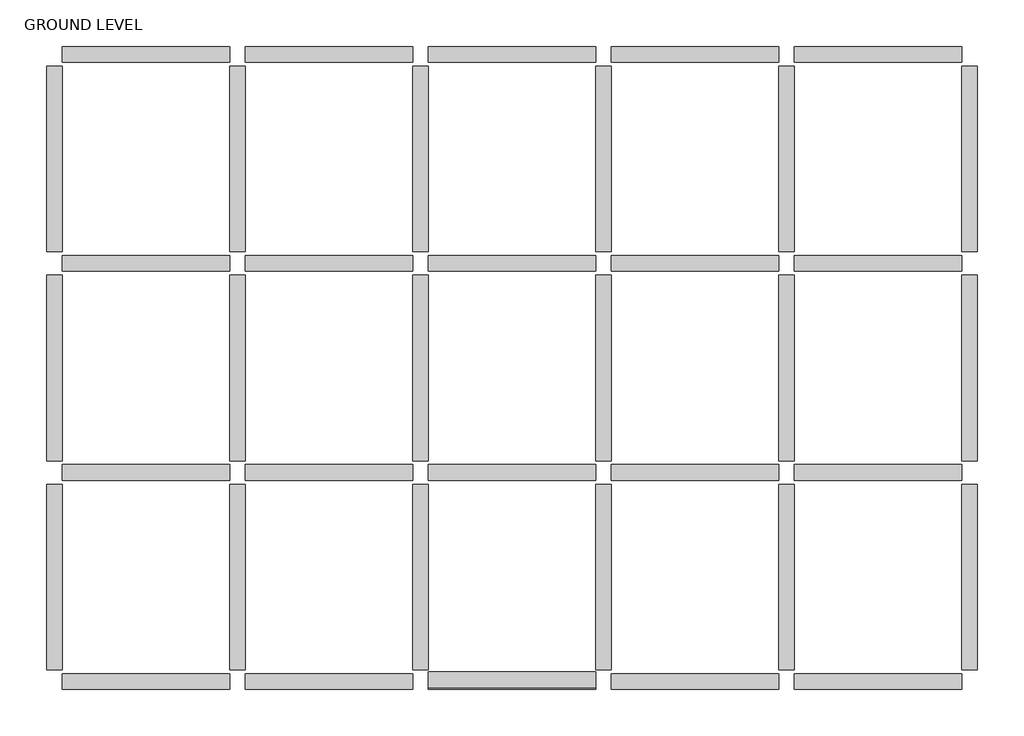
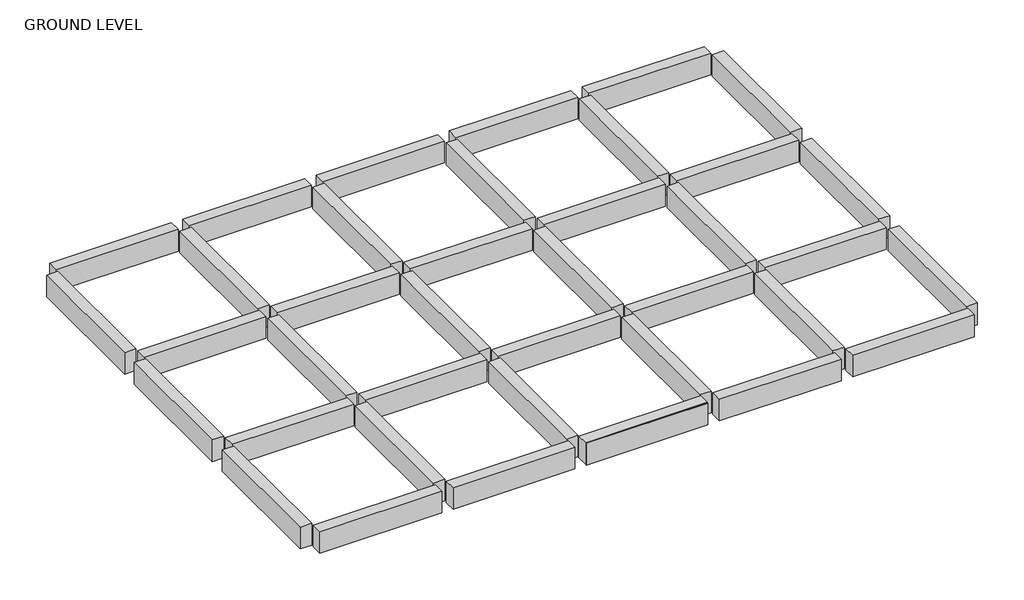
# One storey: 39 beams.
"""IFC4 building model written with IfcOpenShell, lengths in millimetres."""

from ifc_helpers import new_model, si_unit, frame, origin, place, context, project, spatial, polyline, outline, extrude, element, save

model = new_model("IFC4")

# Units and contexts
model_context = context("Model", 3, world=origin())
ifc_project = project(units=[si_unit("LENGTHUNIT", "METRE", prefix="MILLI")], contexts=[model_context])

# Site, building, storey
site = spatial("IfcSite", under=ifc_project)
building = spatial("IfcBuilding", under=site)
storey = spatial("IfcBuildingStorey", under=building, Name="GROUND LEVEL", Elevation=0.0)

# Beams
placement = place(None, origin())
element("IfcBeam", 1, ObjectType="M_Concrete-Rectangular Beam : 300 x 600mm", at=placement, inside=storey, context=model_context, shape_type="SweptSolid", body=[
    extrude(outline(polyline([(-8225.6838695, 13443.2036311), (-8525.6838695, 13443.2036311), (-8525.6838695, 16993.2036311), (-8225.6838695, 16993.2036311), (-8225.6838695, 13443.2036311)])), frame((0.0, 0.0, -600.0), z_axis=(0.0, 0.0, 1.0), x_axis=(1.0, 0.0, 0.0)), (0.0, 0.0, 1.0), 600.0),
])
element("IfcBeam", 2, ObjectType="M_Concrete-Rectangular Beam : 300 x 600mm", at=placement, inside=storey, context=model_context, shape_type="SweptSolid", body=[
    extrude(outline(polyline([(-8525.6838695, 12993.2036311), (-8225.6838695, 12993.2036311), (-8225.6838695, 9443.2036311), (-8525.6838695, 9443.2036311), (-8525.6838695, 12993.2036311)])), frame((0.0, 0.0, -600.0), z_axis=(0.0, 0.0, 1.0), x_axis=(1.0, 0.0, 0.0)), (0.0, 0.0, 1.0), 600.0),
])
element("IfcBeam", 3, ObjectType="M_Concrete-Rectangular Beam : 300 x 600mm", at=placement, inside=storey, context=model_context, shape_type="SweptSolid", body=[
    extrude(outline(polyline([(-8225.6838695, 5443.2036311), (-8525.6838695, 5443.2036311), (-8525.6838695, 8993.2036311), (-8225.6838695, 8993.2036311), (-8225.6838695, 5443.2036311)])), frame((0.0, 0.0, -600.0), z_axis=(0.0, 0.0, 1.0), x_axis=(1.0, 0.0, 0.0)), (0.0, 0.0, 1.0), 600.0),
])
element("IfcBeam", 4, ObjectType="M_Concrete-Rectangular Beam : 300 x 600mm", at=placement, inside=storey, context=model_context, shape_type="SweptSolid", body=[
    extrude(outline(polyline([(-5025.6838695, 5368.2036311), (-5025.6838695, 5068.2036311), (-8225.6838695, 5068.2036311), (-8225.6838695, 5368.2036311), (-5025.6838695, 5368.2036311)])), frame((0.0, 0.0, -600.0), z_axis=(0.0, 0.0, 1.0), x_axis=(1.0, 0.0, 0.0)), (0.0, 0.0, 1.0), 600.0),
])
element("IfcBeam", 5, ObjectType="M_Concrete-Rectangular Beam : 300 x 600mm", at=placement, inside=storey, context=model_context, shape_type="SweptSolid", body=[
    extrude(outline(polyline([(-1525.6838695, 5368.2036311), (-1525.6838695, 5068.2036311), (-4725.6838695, 5068.2036311), (-4725.6838695, 5368.2036311), (-1525.6838695, 5368.2036311)])), frame((0.0, 0.0, -600.0), z_axis=(0.0, 0.0, 1.0), x_axis=(1.0, 0.0, 0.0)), (0.0, 0.0, 1.0), 600.0),
])
element("IfcBeam", 6, ObjectType="M_Concrete-Rectangular Beam : 300 x 600mm", at=placement, inside=storey, context=model_context, shape_type="SweptSolid", body=[
    extrude(outline(polyline([(1974.3161305, 5399.3942253), (1974.3161305, 5099.3942253), (-1225.6838695, 5099.3942253), (-1225.6838695, 5399.3942253), (1974.3161305, 5399.3942253)])), frame((0.0, 0.0, -600.0), z_axis=(0.0, 0.0, 1.0), x_axis=(1.0, 0.0, 0.0)), (0.0, 0.0, 1.0), 600.0),
])
element("IfcBeam", 7, ObjectType="M_Concrete-Rectangular Beam : 300 x 600mm", at=placement, inside=storey, context=model_context, shape_type="SweptSolid", body=[
    extrude(outline(polyline([(-5025.6838695, 8993.2036311), (-4725.6838695, 8993.2036311), (-4725.6838695, 5443.2036311), (-5025.6838695, 5443.2036311), (-5025.6838695, 8993.2036311)])), frame((0.0, 0.0, -600.0), z_axis=(0.0, 0.0, 1.0), x_axis=(1.0, 0.0, 0.0)), (0.0, 0.0, 1.0), 600.0),
])
element("IfcBeam", 8, ObjectType="M_Concrete-Rectangular Beam : 300 x 600mm", at=placement, inside=storey, context=model_context, shape_type="SweptSolid", body=[
    extrude(outline(polyline([(-5025.6838695, 12993.2036311), (-4725.6838695, 12993.2036311), (-4725.6838695, 9443.2036311), (-5025.6838695, 9443.2036311), (-5025.6838695, 12993.2036311)])), frame((0.0, 0.0, -600.0), z_axis=(0.0, 0.0, 1.0), x_axis=(1.0, 0.0, 0.0)), (0.0, 0.0, 1.0), 600.0),
])
element("IfcBeam", 9, ObjectType="M_Concrete-Rectangular Beam : 300 x 600mm", at=placement, inside=storey, context=model_context, shape_type="SweptSolid", body=[
    extrude(outline(polyline([(-5025.6838695, 16993.2036311), (-4725.6838695, 16993.2036311), (-4725.6838695, 13443.2036311), (-5025.6838695, 13443.2036311), (-5025.6838695, 16993.2036311)])), frame((0.0, 0.0, -600.0), z_axis=(0.0, 0.0, 1.0), x_axis=(1.0, 0.0, 0.0)), (0.0, 0.0, 1.0), 600.0),
])
element("IfcBeam", 10, ObjectType="M_Concrete-Rectangular Beam : 300 x 600mm", at=placement, inside=storey, context=model_context, shape_type="SweptSolid", body=[
    extrude(outline(polyline([(-1525.6838695, 8993.2036311), (-1225.6838695, 8993.2036311), (-1225.6838695, 5443.2036311), (-1525.6838695, 5443.2036311), (-1525.6838695, 8993.2036311)])), frame((0.0, 0.0, -600.0), z_axis=(0.0, 0.0, 1.0), x_axis=(1.0, 0.0, 0.0)), (0.0, 0.0, 1.0), 600.0),
])
element("IfcBeam", 11, ObjectType="M_Concrete-Rectangular Beam : 300 x 600mm", at=placement, inside=storey, context=model_context, shape_type="SweptSolid", body=[
    extrude(outline(polyline([(-1525.6838695, 12993.2036311), (-1225.6838695, 12993.2036311), (-1225.6838695, 9443.2036311), (-1525.6838695, 9443.2036311), (-1525.6838695, 12993.2036311)])), frame((0.0, 0.0, -600.0), z_axis=(0.0, 0.0, 1.0), x_axis=(1.0, 0.0, 0.0)), (0.0, 0.0, 1.0), 600.0),
])
element("IfcBeam", 12, ObjectType="M_Concrete-Rectangular Beam : 300 x 600mm", at=placement, inside=storey, context=model_context, shape_type="SweptSolid", body=[
    extrude(outline(polyline([(-1525.6838695, 16993.2036311), (-1225.6838695, 16993.2036311), (-1225.6838695, 13443.2036311), (-1525.6838695, 13443.2036311), (-1525.6838695, 16993.2036311)])), frame((0.0, 0.0, -600.0), z_axis=(0.0, 0.0, 1.0), x_axis=(1.0, 0.0, 0.0)), (0.0, 0.0, 1.0), 600.0),
])
element("IfcBeam", 13, ObjectType="M_Concrete-Rectangular Beam : 300 x 600mm", at=placement, inside=storey, context=model_context, shape_type="SweptSolid", body=[
    extrude(outline(polyline([(1974.3161305, 8993.2036311), (2274.3161305, 8993.2036311), (2274.3161305, 5443.2036311), (1974.3161305, 5443.2036311), (1974.3161305, 8993.2036311)])), frame((0.0, 0.0, -600.0), z_axis=(0.0, 0.0, 1.0), x_axis=(1.0, 0.0, 0.0)), (0.0, 0.0, 1.0), 600.0),
])
element("IfcBeam", 14, ObjectType="M_Concrete-Rectangular Beam : 300 x 600mm", at=placement, inside=storey, context=model_context, shape_type="SweptSolid", body=[
    extrude(outline(polyline([(1974.3161305, 12993.2036311), (2274.3161305, 12993.2036311), (2274.3161305, 9443.2036311), (1974.3161305, 9443.2036311), (1974.3161305, 12993.2036311)])), frame((0.0, 0.0, -600.0), z_axis=(0.0, 0.0, 1.0), x_axis=(1.0, 0.0, 0.0)), (0.0, 0.0, 1.0), 600.0),
])
element("IfcBeam", 15, ObjectType="M_Concrete-Rectangular Beam : 300 x 600mm", at=placement, inside=storey, context=model_context, shape_type="SweptSolid", body=[
    extrude(outline(polyline([(1974.3161305, 16993.2036311), (2274.3161305, 16993.2036311), (2274.3161305, 13443.2036311), (1974.3161305, 13443.2036311), (1974.3161305, 16993.2036311)])), frame((0.0, 0.0, -600.0), z_axis=(0.0, 0.0, 1.0), x_axis=(1.0, 0.0, 0.0)), (0.0, 0.0, 1.0), 600.0),
])
element("IfcBeam", 16, ObjectType="M_Concrete-Rectangular Beam : 300 x 600mm", at=placement, inside=storey, context=model_context, shape_type="SweptSolid", body=[
    extrude(outline(polyline([(5474.3161305, 8993.2036311), (5774.3161305, 8993.2036311), (5774.3161305, 5443.2036311), (5474.3161305, 5443.2036311), (5474.3161305, 8993.2036311)])), frame((0.0, 0.0, -600.0), z_axis=(0.0, 0.0, 1.0), x_axis=(1.0, 0.0, 0.0)), (0.0, 0.0, 1.0), 600.0),
])
element("IfcBeam", 17, ObjectType="M_Concrete-Rectangular Beam : 300 x 600mm", at=placement, inside=storey, context=model_context, shape_type="SweptSolid", body=[
    extrude(outline(polyline([(5474.3161305, 12993.2036311), (5774.3161305, 12993.2036311), (5774.3161305, 9443.2036311), (5474.3161305, 9443.2036311), (5474.3161305, 12993.2036311)])), frame((0.0, 0.0, -600.0), z_axis=(0.0, 0.0, 1.0), x_axis=(1.0, 0.0, 0.0)), (0.0, 0.0, 1.0), 600.0),
])
element("IfcBeam", 18, ObjectType="M_Concrete-Rectangular Beam : 300 x 600mm", at=placement, inside=storey, context=model_context, shape_type="SweptSolid", body=[
    extrude(outline(polyline([(5474.3161305, 16993.2036311), (5774.3161305, 16993.2036311), (5774.3161305, 13443.2036311), (5474.3161305, 13443.2036311), (5474.3161305, 16993.2036311)])), frame((0.0, 0.0, -600.0), z_axis=(0.0, 0.0, 1.0), x_axis=(1.0, 0.0, 0.0)), (0.0, 0.0, 1.0), 600.0),
])
element("IfcBeam", 19, ObjectType="M_Concrete-Rectangular Beam : 300 x 600mm", at=placement, inside=storey, context=model_context, shape_type="SweptSolid", body=[
    extrude(outline(polyline([(8974.3161305, 8993.2036311), (9274.3161305, 8993.2036311), (9274.3161305, 5443.2036311), (8974.3161305, 5443.2036311), (8974.3161305, 8993.2036311)])), frame((0.0, 0.0, -600.0), z_axis=(0.0, 0.0, 1.0), x_axis=(1.0, 0.0, 0.0)), (0.0, 0.0, 1.0), 600.0),
])
element("IfcBeam", 20, ObjectType="M_Concrete-Rectangular Beam : 300 x 600mm", at=placement, inside=storey, context=model_context, shape_type="SweptSolid", body=[
    extrude(outline(polyline([(8974.3161305, 12993.2036311), (9274.3161305, 12993.2036311), (9274.3161305, 9443.2036311), (8974.3161305, 9443.2036311), (8974.3161305, 12993.2036311)])), frame((0.0, 0.0, -600.0), z_axis=(0.0, 0.0, 1.0), x_axis=(1.0, 0.0, 0.0)), (0.0, 0.0, 1.0), 600.0),
])
element("IfcBeam", 21, ObjectType="M_Concrete-Rectangular Beam : 300 x 600mm", at=placement, inside=storey, context=model_context, shape_type="SweptSolid", body=[
    extrude(outline(polyline([(8974.3161305, 16993.2036311), (9274.3161305, 16993.2036311), (9274.3161305, 13443.2036311), (8974.3161305, 13443.2036311), (8974.3161305, 16993.2036311)])), frame((0.0, 0.0, -600.0), z_axis=(0.0, 0.0, 1.0), x_axis=(1.0, 0.0, 0.0)), (0.0, 0.0, 1.0), 600.0),
])
element("IfcBeam", 22, ObjectType="M_Concrete-Rectangular Beam : 300 x 600mm", at=placement, inside=storey, context=model_context, shape_type="SweptSolid", body=[
    extrude(outline(polyline([(-8225.6838695, 17068.2036311), (-8225.6838695, 17368.2036311), (-5025.6838695, 17368.2036311), (-5025.6838695, 17068.2036311), (-8225.6838695, 17068.2036311)])), frame((0.0, 0.0, -600.0), z_axis=(0.0, 0.0, 1.0), x_axis=(1.0, 0.0, 0.0)), (0.0, 0.0, 1.0), 600.0),
])
element("IfcBeam", 23, ObjectType="M_Concrete-Rectangular Beam : 300 x 600mm", at=placement, inside=storey, context=model_context, shape_type="SweptSolid", body=[
    extrude(outline(polyline([(-4725.6838695, 17068.2036311), (-4725.6838695, 17368.2036311), (-1525.6838695, 17368.2036311), (-1525.6838695, 17068.2036311), (-4725.6838695, 17068.2036311)])), frame((0.0, 0.0, -600.0), z_axis=(0.0, 0.0, 1.0), x_axis=(1.0, 0.0, 0.0)), (0.0, 0.0, 1.0), 600.0),
])
element("IfcBeam", 24, ObjectType="M_Concrete-Rectangular Beam : 300 x 600mm", at=placement, inside=storey, context=model_context, shape_type="SweptSolid", body=[
    extrude(outline(polyline([(-1225.6838695, 17068.2036311), (-1225.6838695, 17368.2036311), (1974.3161305, 17368.2036311), (1974.3161305, 17068.2036311), (-1225.6838695, 17068.2036311)])), frame((0.0, 0.0, -600.0), z_axis=(0.0, 0.0, 1.0), x_axis=(1.0, 0.0, 0.0)), (0.0, 0.0, 1.0), 600.0),
])
element("IfcBeam", 25, ObjectType="M_Concrete-Rectangular Beam : 300 x 600mm", at=placement, inside=storey, context=model_context, shape_type="SweptSolid", body=[
    extrude(outline(polyline([(2274.3161305, 17068.2036311), (2274.3161305, 17368.2036311), (5474.3161305, 17368.2036311), (5474.3161305, 17068.2036311), (2274.3161305, 17068.2036311)])), frame((0.0, 0.0, -600.0), z_axis=(0.0, 0.0, 1.0), x_axis=(1.0, 0.0, 0.0)), (0.0, 0.0, 1.0), 600.0),
])
element("IfcBeam", 26, ObjectType="M_Concrete-Rectangular Beam : 300 x 600mm", at=placement, inside=storey, context=model_context, shape_type="SweptSolid", body=[
    extrude(outline(polyline([(5774.3161305, 17068.2036311), (5774.3161305, 17368.2036311), (8974.3161305, 17368.2036311), (8974.3161305, 17068.2036311), (5774.3161305, 17068.2036311)])), frame((0.0, 0.0, -600.0), z_axis=(0.0, 0.0, 1.0), x_axis=(1.0, 0.0, 0.0)), (0.0, 0.0, 1.0), 600.0),
])
element("IfcBeam", 27, ObjectType="M_Concrete-Rectangular Beam : 300 x 600mm", at=placement, inside=storey, context=model_context, shape_type="SweptSolid", body=[
    extrude(outline(polyline([(-5025.6838695, 13368.2036311), (-5025.6838695, 13068.2036311), (-8225.6838695, 13068.2036311), (-8225.6838695, 13368.2036311), (-5025.6838695, 13368.2036311)])), frame((0.0, 0.0, -600.0), z_axis=(0.0, 0.0, 1.0), x_axis=(1.0, 0.0, 0.0)), (0.0, 0.0, 1.0), 600.0),
])
element("IfcBeam", 28, ObjectType="M_Concrete-Rectangular Beam : 300 x 600mm", at=placement, inside=storey, context=model_context, shape_type="SweptSolid", body=[
    extrude(outline(polyline([(-1525.6838695, 13368.2036311), (-1525.6838695, 13068.2036311), (-4725.6838695, 13068.2036311), (-4725.6838695, 13368.2036311), (-1525.6838695, 13368.2036311)])), frame((0.0, 0.0, -600.0), z_axis=(0.0, 0.0, 1.0), x_axis=(1.0, 0.0, 0.0)), (0.0, 0.0, 1.0), 600.0),
])
element("IfcBeam", 29, ObjectType="M_Concrete-Rectangular Beam : 300 x 600mm", at=placement, inside=storey, context=model_context, shape_type="SweptSolid", body=[
    extrude(outline(polyline([(1974.3161305, 13368.2036311), (1974.3161305, 13068.2036311), (-1225.6838695, 13068.2036311), (-1225.6838695, 13368.2036311), (1974.3161305, 13368.2036311)])), frame((0.0, 0.0, -600.0), z_axis=(0.0, 0.0, 1.0), x_axis=(1.0, 0.0, 0.0)), (0.0, 0.0, 1.0), 600.0),
])
element("IfcBeam", 30, ObjectType="M_Concrete-Rectangular Beam : 300 x 600mm", at=placement, inside=storey, context=model_context, shape_type="SweptSolid", body=[
    extrude(outline(polyline([(5474.3161305, 13368.2036311), (5474.3161305, 13068.2036311), (2274.3161305, 13068.2036311), (2274.3161305, 13368.2036311), (5474.3161305, 13368.2036311)])), frame((0.0, 0.0, -600.0), z_axis=(0.0, 0.0, 1.0), x_axis=(1.0, 0.0, 0.0)), (0.0, 0.0, 1.0), 600.0),
])
element("IfcBeam", 31, ObjectType="M_Concrete-Rectangular Beam : 300 x 600mm", at=placement, inside=storey, context=model_context, shape_type="SweptSolid", body=[
    extrude(outline(polyline([(8974.3161305, 13368.2036311), (8974.3161305, 13068.2036311), (5774.3161305, 13068.2036311), (5774.3161305, 13368.2036311), (8974.3161305, 13368.2036311)])), frame((0.0, 0.0, -600.0), z_axis=(0.0, 0.0, 1.0), x_axis=(1.0, 0.0, 0.0)), (0.0, 0.0, 1.0), 600.0),
])
element("IfcBeam", 32, ObjectType="M_Concrete-Rectangular Beam : 300 x 600mm", at=placement, inside=storey, context=model_context, shape_type="SweptSolid", body=[
    extrude(outline(polyline([(-8225.6838695, 9068.2036311), (-8225.6838695, 9368.2036311), (-5025.6838695, 9368.2036311), (-5025.6838695, 9068.2036311), (-8225.6838695, 9068.2036311)])), frame((0.0, 0.0, -600.0), z_axis=(0.0, 0.0, 1.0), x_axis=(1.0, 0.0, 0.0)), (0.0, 0.0, 1.0), 600.0),
])
element("IfcBeam", 33, ObjectType="M_Concrete-Rectangular Beam : 300 x 600mm", at=placement, inside=storey, context=model_context, shape_type="SweptSolid", body=[
    extrude(outline(polyline([(-4725.6838695, 9068.2036311), (-4725.6838695, 9368.2036311), (-1525.6838695, 9368.2036311), (-1525.6838695, 9068.2036311), (-4725.6838695, 9068.2036311)])), frame((0.0, 0.0, -600.0), z_axis=(0.0, 0.0, 1.0), x_axis=(1.0, 0.0, 0.0)), (0.0, 0.0, 1.0), 600.0),
])
element("IfcBeam", 34, ObjectType="M_Concrete-Rectangular Beam : 300 x 600mm", at=placement, inside=storey, context=model_context, shape_type="SweptSolid", body=[
    extrude(outline(polyline([(-1225.6838695, 9068.2036311), (-1225.6838695, 9368.2036311), (1974.3161305, 9368.2036311), (1974.3161305, 9068.2036311), (-1225.6838695, 9068.2036311)])), frame((0.0, 0.0, -600.0), z_axis=(0.0, 0.0, 1.0), x_axis=(1.0, 0.0, 0.0)), (0.0, 0.0, 1.0), 600.0),
])
element("IfcBeam", 35, ObjectType="M_Concrete-Rectangular Beam : 300 x 600mm", at=placement, inside=storey, context=model_context, shape_type="SweptSolid", body=[
    extrude(outline(polyline([(2274.3161305, 9068.2036311), (2274.3161305, 9368.2036311), (5474.3161305, 9368.2036311), (5474.3161305, 9068.2036311), (2274.3161305, 9068.2036311)])), frame((0.0, 0.0, -600.0), z_axis=(0.0, 0.0, 1.0), x_axis=(1.0, 0.0, 0.0)), (0.0, 0.0, 1.0), 600.0),
])
element("IfcBeam", 36, ObjectType="M_Concrete-Rectangular Beam : 300 x 600mm", at=placement, inside=storey, context=model_context, shape_type="SweptSolid", body=[
    extrude(outline(polyline([(5774.3161305, 9068.2036311), (5774.3161305, 9368.2036311), (8974.3161305, 9368.2036311), (8974.3161305, 9068.2036311), (5774.3161305, 9068.2036311)])), frame((0.0, 0.0, -600.0), z_axis=(0.0, 0.0, 1.0), x_axis=(1.0, 0.0, 0.0)), (0.0, 0.0, 1.0), 600.0),
])
element("IfcBeam", 37, ObjectType="M_Concrete-Rectangular Beam : 300 x 600mm", at=placement, inside=storey, context=model_context, shape_type="SweptSolid", body=[
    extrude(outline(polyline([(1974.3161305, 5068.2036311), (-1225.6838695, 5068.2036311), (-1225.6838695, 5099.3942253), (1974.3161305, 5099.3942253), (1974.3161305, 5068.2036311)])), frame((0.0, 0.0, -600.0), z_axis=(0.0, 0.0, 1.0), x_axis=(1.0, 0.0, 0.0)), (0.0, 0.0, 1.0), 600.0),
])
element("IfcBeam", 38, ObjectType="M_Concrete-Rectangular Beam : 300 x 600mm", at=placement, inside=storey, context=model_context, shape_type="SweptSolid", body=[
    extrude(outline(polyline([(5474.3161305, 5368.2036311), (5474.3161305, 5068.2036311), (2274.3161305, 5068.2036311), (2274.3161305, 5368.2036311), (5474.3161305, 5368.2036311)])), frame((0.0, 0.0, -600.0), z_axis=(0.0, 0.0, 1.0), x_axis=(1.0, 0.0, 0.0)), (0.0, 0.0, 1.0), 600.0),
])
element("IfcBeam", 39, ObjectType="M_Concrete-Rectangular Beam : 300 x 600mm", at=placement, inside=storey, context=model_context, shape_type="SweptSolid", body=[
    extrude(outline(polyline([(8974.3161305, 5368.2036311), (8974.3161305, 5068.2036311), (5774.3161305, 5068.2036311), (5774.3161305, 5368.2036311), (8974.3161305, 5368.2036311)])), frame((0.0, 0.0, -600.0), z_axis=(0.0, 0.0, 1.0), x_axis=(1.0, 0.0, 0.0)), (0.0, 0.0, 1.0), 600.0),
])

save(model, "model.ifc")

# Revit data of these elements
# Type "M_Concrete-Rectangular Beam : 300 x 600mm"
#   Length [instance default] = 1524 mm
#   b = 300 mm
#   h = 600 mm
#   Structural Material [instance default] = Concrete, Cast-in-Place gray
#   Assembly Code = ""
# Elements 1, 2, 3, 4, 5, 6, 7, 8, 9, 10, 11, 12, 13, 14, 15, 16, 17, 18, 19, 20, 21, 22, 23, 24, 25, 26, 27, 28, 29, 30, 31, 32, 33, 34, 35, 36, 37, 38, 39 (IfcBeam, "M_Concrete-Rectangular Beam : 300 x 600mm")
#   Structural Material = Concrete, Cast-in-Place gray
#   Phase Created = New Construction
#   Materials on its faces: "Concrete, Cast-in-Place gray"
# Materials
#   "Concrete, Cast-in-Place gray": class "Concrete", colour RGB 192 192 192, transparency 0, Description = "Cast-in-place concrete", Cost = 0
